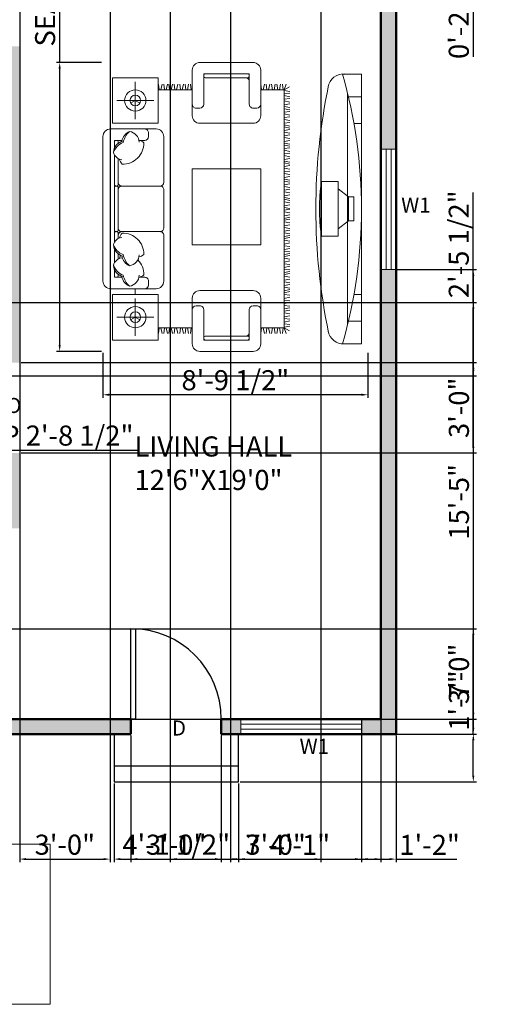
# Model space of a CAD drawing. Units: inches. Extents: x 3655 to 4051, y 2160 to 2854.
# Tile 2 of 3: x 3863 to 4051, y 2160 to 2552. Entities that reach past the tile are written whole.
import ezdxf

# ---------------------------------------------------------------- set-up
doc = ezdxf.new("R2010")
doc.units = ezdxf.units.IN
for name, color, linetype, lineweight in [('A-ANNO-DIMS', 2, 'Continuous', 18), ('A-ANNO-SCHD', 7, 'Continuous', 18), ('A-ANNO-TEXT', 7, 'Continuous', 18), ('A-AREA-IDEN', 7, 'Continuous', 25), ('A-DOOR', 3, 'Continuous', 25), ('A-FLOR-STRS', 7, 'Continuous', 25), ('A-FURN', 8, 'Continuous', 18), ('A-GLAZ', 4, 'Continuous', 18), ('A-WALL', 7, 'Continuous', 50)]:
    doc.layers.add(name, color=color, linetype=linetype, lineweight=lineweight)
doc.layers.add('A-WALL-PATT', color=244, linetype='Continuous', lineweight=13, true_color=0x991b1e)
doc.styles.get("Standard").update_dxf_attribs({"font": 'arial.ttf'})
doc.dimstyles.new('ISO-25', dxfattribs={"dimtxt": 8, "dimasz": 2.5, "dimexe": 1.25, "dimexo": 0.625, "dimtad": 1, "dimdec": 1, "dimlunit": 3, "dimtxsty": 'Standard', "dimcen": 2.5, "dimadec": 0, "dimazin": 0, "dimtfac": 1, "dimtdec": 1, "dimtmove": 0, "dimatfit": 3, "dimfxl": 1, "dimarcsym": 0})

# ---------------------------------------------------------------- blocks, each defined once
blk = doc.blocks.new('*U2')
for p, q in [((0, 0), (0, -6)), ((36, 0), (36, -6))]:
    blk.add_line(p, q)
blk.add_lwpolyline([(0, 0), (0, 36), (1.75, 36), (1.75, 0)], close=True)
blk.add_arc((0, 0), 36, 0, 90)
blk = doc.blocks.new('A$C78AE5658')
for p, q in [((925, 3400), (2825, 3400)), ((150, 3275), (150, 2675)), ((750, 3275), (150, 3275)), ((750, 2675), (750, 3275)), ((825, 2700), (825, 3300)), ((975, 3250), (975, 3152)), ((1080, 3250), (975, 3250)), ((995, 3250), (1080, 3250)), ((1163, 3250), (1350, 3250)), ((1350, 3250), (1163, 3250)), ((2587, 3250), (1433, 3250)), ((1433, 3250), (1555, 3250)), ((1595, 3250), (2155, 3250)), ((2587, 3250), (2195, 3250)), ((2775, 3250), (2670, 3250)), ((2755, 3250), (2670, 3250)), ((2775, 3152), (2775, 3250)), ((2925, 3300), (2925, 2700)), ((3000, 3275), (3000, 2675)), ((3600, 3275), (3000, 3275)), ((3600, 2675), (3600, 3275)), ((450, 2730), (450, 3220)), ((975, 3220), (975, 3230)), ((1013, 3200), (995, 3200)), ((1283, 3200), (1214, 3200)), ((1555, 3200), (1483, 3200)), ((1575, 3230), (1575, 3220)), ((1575, 3220), (1575, 3230)), ((1575, 3150), (1575, 2650)), ((2155, 3200), (1595, 3200)), ((2175, 3230), (2175, 3220)), ((2175, 3230), (2175, 3220)), ((2175, 3150), (2175, 2650)), ((2195, 3200), (2536, 3200)), ((2737, 3200), (2755, 3200)), ((2775, 3220), (2775, 3230)), ((3300, 2730), (3300, 3220)), ((450, 2975), (415, 3036)), ((3300, 2975), (3265, 3036)), ((205, 2975), (695, 2975)), ((450, 2975), (415, 2914)), ((750, 2975), (825, 2975)), ((975, 2927), (975, 2850)), ((2775, 2850), (2775, 2927)), ((3055, 2975), (3545, 2975)), ((3300, 2975), (3265, 2914)), ((925, 2800), (875, 2800)), ((2875, 2800), (2825, 2800)), ((150, 2675), (750, 2675)), ((308, 2659), (234, 2670)), ((308, 2637), (234, 2622)), ((308, 2589), (234, 2600)), ((308, 2675), (308, 2225)), ((1525, 2600), (925, 2600)), ((2125, 2600), (1625, 2600)), ((2825, 2600), (2225, 2600)), ((3000, 2675), (3600, 2675)), ((3442, 2675), (3442, 2225)), ((3442, 2659), (3516, 2670)), ((3442, 2637), (3516, 2622)), ((3442, 2589), (3516, 2600)), ((308, 2567), (234, 2552)), ((308, 2524), (234, 2535)), ((308, 2501), (234, 2487)), ((308, 2453), (234, 2464)), ((3442, 2567), (3516, 2552)), ((3442, 2524), (3516, 2535)), ((3442, 2501), (3516, 2487)), ((3442, 2453), (3516, 2464)), ((308, 2431), (234, 2417)), ((308, 2380), (234, 2391)), ((308, 2357), (234, 2343)), ((3442, 2431), (3516, 2417)), ((3442, 2380), (3516, 2391)), ((3442, 2357), (3516, 2343)), ((100, 2225), (700, 2225)), ((308, 2310), (234, 2321)), ((308, 2288), (234, 2273)), ((308, 2238), (234, 2249)), ((1400, 2225), (1400, 1325)), ((2400, 2225), (1400, 2225)), ((2400, 1325), (2400, 2225)), ((3700, 2225), (3100, 2225)), ((3442, 2310), (3516, 2321)), ((3442, 2288), (3516, 2273)), ((3442, 2238), (3516, 2249)), ((0, 1425), (0, 2125)), ((150, 2075), (150, 1475)), ((550, 2075), (150, 2075)), ((180, 2075), (170, 2075)), ((600, 2125), (600, 2175)), ((800, 2125), (800, 1425)), ((3000, 2125), (3000, 1425)), ((3200, 2125), (3200, 2175)), ((3250, 2075), (3650, 2075)), ((3620, 2075), (3630, 2075)), ((3650, 2075), (3650, 1475)), ((3800, 1425), (3800, 2125)), ((200, 2037), (200, 2055)), ((200, 1495), (200, 2037)), ((3600, 2037), (3600, 2055)), ((3600, 1495), (3600, 2037)), ((150, 1887), (150, 1495)), ((150, 1887), (150, 1475)), ((3650, 1887), (3650, 1495)), ((3650, 1887), (3650, 1475)), ((550, 1475), (150, 1475)), ((150, 1475), (550, 1475)), ((150, 1475), (550, 1475)), ((170, 1475), (180, 1475)), ((170, 1475), (180, 1475)), ((600, 1425), (600, 1375)), ((600, 1425), (600, 1375)), ((3200, 1425), (3200, 1375)), ((3200, 1425), (3200, 1375)), ((3250, 1475), (3650, 1475)), ((3650, 1475), (3250, 1475)), ((3650, 1475), (3250, 1475)), ((3630, 1475), (3620, 1475)), ((3630, 1475), (3620, 1475)), ((700, 1325), (100, 1325)), ((308, 1314), (234, 1325)), ((1400, 1325), (2400, 1325)), ((3100, 1325), (3700, 1325)), ((3442, 1314), (3516, 1325)), ((308, 1291), (234, 1277)), ((308, 1244), (234, 1255)), ((308, 1221), (234, 1207)), ((308, 1170), (234, 1181)), ((3442, 1291), (3516, 1277)), ((3442, 1244), (3516, 1255)), ((3442, 1221), (3516, 1207)), ((3442, 1170), (3516, 1181)), ((308, 1147), (234, 1133)), ((308, 1100), (234, 1111)), ((308, 1078), (234, 1063)), ((308, 1028), (234, 1039)), ((3442, 1147), (3516, 1133)), ((3442, 1100), (3516, 1111)), ((3442, 1078), (3516, 1063)), ((3442, 1028), (3516, 1039)), ((308, 1015), (236, 991)), ((308, 1015), (270, 946)), ((317, 1015), (332, 942)), ((363, 1015), (352, 942)), ((386, 1015), (400, 942)), ((434, 1015), (422, 942)), ((456, 1015), (470, 942)), ((507, 1015), (496, 942)), ((530, 1015), (544, 942)), ((559, 1015), (574, 942)), ((605, 1015), (594, 942)), ((628, 1015), (642, 942)), ((675, 1015), (664, 942)), ((698, 1015), (712, 942)), ((749, 1015), (738, 942)), ((771, 1015), (786, 942)), ((798, 1015), (813, 942)), ((845, 1015), (833, 942)), ((867, 1015), (881, 942)), ((915, 1015), (904, 942)), ((937, 1015), (951, 942)), ((989, 1015), (977, 942)), ((1011, 1015), (1025, 942)), ((1036, 1015), (1051, 942)), ((1082, 1015), (1071, 942)), ((1104, 1015), (1119, 942)), ((1152, 1015), (1141, 942)), ((1175, 1015), (1189, 942)), ((1226, 1015), (1215, 942)), ((1248, 1015), (1263, 942)), ((1273, 1015), (1287, 942)), ((1319, 1015), (1308, 942)), ((1341, 1015), (1355, 942)), ((1389, 1015), (1378, 942)), ((1411, 1015), (1426, 942)), ((1463, 1015), (1452, 942)), ((1485, 1015), (1499, 942)), ((1512, 1015), (1526, 942)), ((1558, 1015), (1547, 942)), ((1580, 1015), (1595, 942)), ((1628, 1015), (1617, 942)), ((1650, 1015), (1665, 942)), ((1702, 1015), (1691, 942)), ((1724, 1015), (1739, 942)), ((1750, 1015), (1764, 942)), ((1783, 1015), (1797, 942)), ((1834, 1015), (1823, 942)), ((1857, 1015), (1871, 942)), ((1894, 1015), (1879, 942)), ((1916, 1015), (1927, 942)), ((1967, 1015), (1953, 942)), ((2000, 1015), (1986, 942)), ((2026, 1015), (2012, 942)), ((2048, 1015), (2059, 942)), ((2100, 1015), (2085, 942)), ((2122, 1015), (2133, 942)), ((2170, 1015), (2155, 942)), ((2192, 1015), (2203, 942)), ((2238, 1015), (2224, 942)), ((2265, 1015), (2251, 942)), ((2288, 1015), (2299, 942)), ((2339, 1015), (2325, 942)), ((2361, 1015), (2372, 942)), ((2409, 1015), (2395, 942)), ((2431, 1015), (2443, 942)), ((2478, 1015), (2463, 942)), ((2502, 1015), (2487, 942)), ((2524, 1015), (2535, 942)), ((2576, 1015), (2561, 942)), ((2598, 1015), (2609, 942)), ((2646, 1015), (2631, 942)), ((2668, 1015), (2679, 942)), ((2714, 1015), (2700, 942)), ((2739, 1015), (2725, 942)), ((2762, 1015), (2773, 942)), ((2813, 1015), (2799, 942)), ((2835, 1015), (2847, 942)), ((2883, 1015), (2869, 942)), ((2906, 1015), (2917, 942)), ((2952, 1015), (2937, 942)), ((2979, 1015), (2964, 942)), ((3001, 1015), (3012, 942)), ((3052, 1015), (3038, 942)), ((3075, 1015), (3086, 942)), ((3123, 1015), (3108, 942)), ((3145, 1015), (3156, 942)), ((3191, 1015), (3177, 942)), ((3221, 1015), (3206, 942)), ((3243, 1015), (3254, 942)), ((3294, 1015), (3280, 942)), ((3317, 1015), (3328, 942)), ((3365, 1015), (3350, 942)), ((3387, 1015), (3398, 942)), ((3433, 1015), (3418, 942)), ((3442, 1015), (3515, 991)), ((3442, 1015), (3480, 946)), ((1515, 306), (1515, 524)), ((1515, 524), (2236, 524)), ((2236, 306), (2236, 524)), ((1515, 306), (2236, 306)), ((1613, 306), (1716, 168)), ((2137, 306), (2034, 168)), ((98, 250), (98, 252)), ((98, 250), (98, 0)), ((348, 184), (3398, 184)), ((398, 0), (398, 172)), ((2034, 168), (1716, 168)), ((1716, 168), (1716, 98)), ((2034, 168), (2034, 98)), ((3348, 0), (3348, 172)), ((3648, 250), (3648, 252)), ((3648, 0), (3648, 250)), ((3648, 0), (98, 0)), ((748, 0), (748, 99)), ((2034, 98), (1716, 98)), ((2998, 0), (2998, 99))]:
    blk.add_line(p, q)
for points in [[(308, 1325), (308, 1015), (1875, 1015)], [(3442, 1325), (3442, 1015), (1875, 1015)]]:
    blk.add_lwpolyline(points)
blk.add_lwpolyline([(246, 432, -0.103184), (3500, 432, -0.103184)], format="xyb")
for centre, radius in [((450, 2975), 140), ((3300, 2975), 140), ((450, 2975), 70), ((3300, 2975), 70)]:
    blk.add_circle(centre, radius)
for centre, radius, start, end in [((925, 3300), 100, 90, 180), ((2825, 3300), 100, 0, 90), ((995, 3230), 20, 90, 180), ((1145, 3093), 170, 94.5332, 162.7286), ((1209, 3055), 221, 110.2594, 158.4317), ((1100, 3136), 130, 7.768, 75.8936), ((1415, 3093), 170, 94.5332, 162.7286), ((1478, 3055), 221, 110.2594, 158.4317), ((1370, 3136), 130, 7.768, 75.8936), ((1555, 3230), 20, 0, 90), ((1595, 3230), 20, 90, 180), ((2155, 3230), 20, 0, 90), ((2195, 3230), 20, 90, 180), ((2650, 3136), 130, 104.1064, 172.232), ((2542, 3055), 221, 21.5683, 69.7406), ((2605, 3093), 170, 17.2714, 85.4668), ((2755, 3230), 20, 0, 90), ((1019, 2980), 177, 100.6387, 156.6848), ((1072, 2852), 293, 103.6492, 137.2632), ((995, 3220), 20, 180, 270), ((1289, 2980), 177, 100.6387, 156.6848), ((1342, 2852), 293, 103.6492, 137.2632), ((1173, 3032), 162, 56.7787, 73.2207), ((1278, 3140), 278, 269.4211, 1.715), ((1443, 3032), 162, 45.5055, 73.2207), ((1525, 3150), 50, 0, 90), ((1555, 3220), 20, 270, 0), ((1595, 3220), 20, 180, 270), ((1625, 3150), 50, 90, 180), ((2125, 3150), 50, 0, 90), ((2155, 3220), 20, 270, 0), ((2195, 3220), 20, 180, 270), ((2225, 3150), 50, 90, 180), ((2577, 3032), 162, 106.7793, 134.4945), ((2741, 3140), 278, 178.285, 270.5789), ((2678, 2852), 293, 42.7368, 76.3508), ((2755, 3220), 20, 270, 0), ((2731, 2980), 177, 23.3152, 79.3613), ((1006, 3075), 151, 189.3928, 267.9328), ((1275, 3075), 151, 189.3928, 267.9328), ((2745, 3075), 151, 272.0672, 350.6072), ((875, 2850), 50, 180, 270), ((925, 2850), 50, 270, 0), ((1088, 2940), 113, 186.2903, 223.8884), ((1009, 3140), 278, 269.4211, 314.7117), ((1357, 2940), 113, 186.2903, 223.8884), ((2663, 2940), 113, 316.1116, 353.7097), ((2825, 2850), 50, 180, 270), ((2875, 2850), 50, 270, 0), ((925, 2700), 100, 180, 270), ((1525, 2650), 50, 270, 0), ((1625, 2650), 50, 180, 270), ((2125, 2650), 50, 270, 0), ((2225, 2650), 50, 180, 270), ((2825, 2700), 100, 270, 0), ((100, 2125), 100, 90, 180), ((550, 2175), 50, 0, 90), ((700, 2125), 100, 0, 90), ((3100, 2125), 100, 90, 180), ((3250, 2175), 50, 90, 180), ((3700, 2125), 100, 0, 90), ((170, 2055), 20, 90, 180), ((180, 2055), 20, 0, 90), ((550, 2125), 50, 270, 0), ((3250, 2125), 50, 180, 270), ((3620, 2055), 20, 90, 180), ((3630, 2055), 20, 0, 90), ((100, 1425), 100, 180, 270), ((170, 1495), 20, 180, 270), ((180, 1495), 20, 270, 0), ((250, 1525), 50, 180, 270), ((550, 1425), 50, 0, 90), ((550, 1425), 50, 0, 90), ((700, 1425), 100, 270, 0), ((3100, 1425), 100, 180, 270), ((3250, 1425), 50, 90, 180), ((3250, 1425), 50, 90, 180), ((3550, 1525), 50, 270, 0), ((3620, 1495), 20, 180, 270), ((3630, 1495), 20, 270, 0), ((3700, 1425), 100, 270, 0), ((550, 1375), 50, 270, 0), ((550, 1375), 50, 270, 0), ((3250, 1375), 50, 180, 270), ((3250, 1375), 50, 180, 270), ((1875, -1675), 2228, 80.6925, 99.3075), ((298, 239), 200, 98.4687, 183.693), ((3449, 239), 200, 356.307, 81.5313), ((1873, 6426), 6426, 253.9658, 286.0342)]:
    blk.add_arc(centre, radius, start, end)
blk = doc.blocks.new('WIN-W1-48IN')
for p, q in [((0, 0), (0, 6)), ((48, 4), (0, 4)), ((48, 0), (48, 6)), ((48, 2), (0, 2))]:
    blk.add_line(p, q)
blk = doc.blocks.new('*D20')
at = {"layer": 'A-ANNO-DIMS', "color": 0, "lineweight": -2, "transparency": 16777216}
for p, q in [((3775.19, 2376.57), (3775.19, 2382.07)), ((3807.66, 2376.57), (3807.66, 2382.07)), ((3777.69, 2380.82), (3805.16, 2380.82)), ((3807.66, 2380.82), (3910.22, 2380.82))]:
    blk.add_line(p, q, dxfattribs=at)
at = {"layer": 'A-ANNO-DIMS', "color": 0, "transparency": 16777216}
for points in [[(3777.69, 2381.24), (3777.69, 2380.4), (3775.19, 2380.82)], [(3805.16, 2381.24), (3805.16, 2380.4), (3807.66, 2380.82)]]:
    blk.add_solid(points, dxfattribs=at)
at = {"layer": 'Defpoints', "color": 0, "transparency": 16777216}
for p in [(3807.66, 2380.82), (3775.19, 2375.95), (3807.66, 2375.95)]:
    blk.add_point(p, dxfattribs=at)
at = {"layer": 'A-ANNO-DIMS', "color": 0, "transparency": 16777216, "insert": (3860.19, 2385.58), "char_height": 8, "attachment_point": 5}
blk.add_mtext('COOKTOP 2\'-8 1/2"', dxfattribs=at)
blk = doc.blocks.new('*D22')
at = {"layer": 'A-ANNO-DIMS', "color": 0, "lineweight": -2, "transparency": 16777216}
for p, q in [((3879.35, 2535.27), (3879.35, 2656.5)), ((3895.99, 2535.27), (3878.1, 2535.27)), ((3879.35, 2422.65), (3879.35, 2532.77)), ((3895.99, 2420.15), (3878.1, 2420.15))]:
    blk.add_line(p, q, dxfattribs=at)
at = {"layer": 'A-ANNO-DIMS', "color": 0, "transparency": 16777216}
for points in [[(3878.93, 2532.77), (3879.76, 2532.77), (3879.35, 2535.27)], [(3878.93, 2422.65), (3879.76, 2422.65), (3879.35, 2420.15)]]:
    blk.add_solid(points, dxfattribs=at)
at = {"layer": 'Defpoints', "color": 0, "transparency": 16777216}
for p in [(3879.35, 2535.27), (3896.61, 2535.27), (3896.61, 2420.15)]:
    blk.add_point(p, dxfattribs=at)
at = {"layer": 'A-ANNO-DIMS', "color": 0, "transparency": 16777216, "insert": (3874.58, 2597.13), "char_height": 8, "attachment_point": 5, "rotation": 90}
blk.add_mtext('SEATING GROUP 9\'-7"', dxfattribs=at)
blk = doc.blocks.new('*D23')
at = {"layer": 'A-ANNO-DIMS', "color": 0, "lineweight": -2, "transparency": 16777216}
for p, q in [((3896.61, 2419.52), (3896.61, 2401.63)), ((4002.13, 2419.52), (4002.13, 2401.63)), ((3999.63, 2402.88), (3899.11, 2402.88))]:
    blk.add_line(p, q, dxfattribs=at)
at = {"layer": 'A-ANNO-DIMS', "color": 0, "transparency": 16777216}
for points in [[(3899.11, 2403.3), (3899.11, 2402.46), (3896.61, 2402.88)], [(3999.63, 2403.3), (3999.63, 2402.46), (4002.13, 2402.88)]]:
    blk.add_solid(points, dxfattribs=at)
at = {"layer": 'Defpoints', "color": 0, "transparency": 16777216}
for p in [(3896.61, 2420.15), (4002.13, 2420.15), (3896.61, 2402.88)]:
    blk.add_point(p, dxfattribs=at)
at = {"layer": 'A-ANNO-DIMS', "color": 0, "transparency": 16777216, "insert": (3949.37, 2407.64), "char_height": 8, "attachment_point": 5}
blk.add_mtext('8\'-9 1/2"', dxfattribs=at)
blk = doc.blocks.new('*D26')
at = {"layer": 'A-ANNO-DIMS', "color": 0, "lineweight": -2, "transparency": 16777216}
for p, q in [((3923.41, 2637.07), (3923.41, 2216.63)), ((4007.41, 2637.07), (4007.41, 2216.63)), ((3925.91, 2217.88), (4004.91, 2217.88))]:
    blk.add_line(p, q, dxfattribs=at)
at = {"layer": 'A-ANNO-DIMS', "color": 0, "transparency": 16777216}
for points in [[(3925.91, 2218.3), (3925.91, 2217.47), (3923.41, 2217.88)], [(4004.91, 2218.3), (4004.91, 2217.47), (4007.41, 2217.88)]]:
    blk.add_solid(points, dxfattribs=at)
at = {"layer": 'Defpoints', "color": 0, "transparency": 16777216}
for p in [(3923.41, 2637.69), (4007.41, 2637.69), (4007.41, 2217.88)]:
    blk.add_point(p, dxfattribs=at)
at = {"layer": 'A-ANNO-DIMS', "color": 0, "transparency": 16777216, "insert": (3965.41, 2222.59), "char_height": 8, "attachment_point": 5}
blk.add_mtext('7\'-0"', dxfattribs=at)
blk = doc.blocks.new('*D28')
at = {"layer": 'A-ANNO-DIMS', "color": 0, "lineweight": -2, "transparency": 16777216}
for p, q in [((3947.41, 2577.07), (3947.41, 2216.63)), ((3983.41, 2577.07), (3983.41, 2216.63)), ((3949.91, 2217.88), (3980.91, 2217.88))]:
    blk.add_line(p, q, dxfattribs=at)
at = {"layer": 'A-ANNO-DIMS', "color": 0, "transparency": 16777216}
for points in [[(3949.91, 2218.3), (3949.91, 2217.47), (3947.41, 2217.88)], [(3980.91, 2218.3), (3980.91, 2217.47), (3983.41, 2217.88)]]:
    blk.add_solid(points, dxfattribs=at)
at = {"layer": 'Defpoints', "color": 0, "transparency": 16777216}
for p in [(3947.41, 2577.69), (3983.41, 2577.69), (3983.41, 2217.88)]:
    blk.add_point(p, dxfattribs=at)
at = {"layer": 'A-ANNO-DIMS', "color": 0, "transparency": 16777216, "insert": (3965.41, 2222.59), "char_height": 8, "attachment_point": 5}
blk.add_mtext('3\'-0"', dxfattribs=at)
blk = doc.blocks.new('*D32')
at = {"layer": 'A-ANNO-DIMS', "color": 0, "lineweight": -2, "transparency": 16777216}
for p, q in [((3864.03, 2415.69), (4045.46, 2415.69)), ((4044.21, 2382.19), (4044.21, 2413.19)), ((3864.03, 2379.69), (4045.46, 2379.69))]:
    blk.add_line(p, q, dxfattribs=at)
at = {"layer": 'A-ANNO-DIMS', "color": 0, "transparency": 16777216}
for points in [[(4043.79, 2413.19), (4044.63, 2413.19), (4044.21, 2415.69)], [(4043.79, 2382.19), (4044.63, 2382.19), (4044.21, 2379.69)]]:
    blk.add_solid(points, dxfattribs=at)
at = {"layer": 'Defpoints', "color": 0, "transparency": 16777216}
for p in [(3863.41, 2415.69), (4044.21, 2415.69), (3863.41, 2379.69)]:
    blk.add_point(p, dxfattribs=at)
at = {"layer": 'A-ANNO-DIMS', "color": 0, "transparency": 16777216, "insert": (4039.5, 2397.69), "char_height": 8, "attachment_point": 5, "rotation": 90}
blk.add_mtext('3\'-0"', dxfattribs=at)
blk = doc.blocks.new('*D33')
at = {"layer": 'A-ANNO-DIMS', "color": 0, "lineweight": -2, "transparency": 16777216}
for p, q in [((3907.77, 2267.07), (3907.77, 2216.63)), ((3943.77, 2267.07), (3943.77, 2216.63)), ((3910.27, 2217.88), (3941.27, 2217.88))]:
    blk.add_line(p, q, dxfattribs=at)
at = {"layer": 'A-ANNO-DIMS', "color": 0, "transparency": 16777216}
for points in [[(3910.27, 2218.3), (3910.27, 2217.47), (3907.77, 2217.88)], [(3941.27, 2218.3), (3941.27, 2217.47), (3943.77, 2217.88)]]:
    blk.add_solid(points, dxfattribs=at)
at = {"layer": 'Defpoints', "color": 0, "transparency": 16777216}
for p in [(3907.77, 2267.69), (3943.77, 2267.69), (3943.77, 2217.88)]:
    blk.add_point(p, dxfattribs=at)
at = {"layer": 'A-ANNO-DIMS', "color": 0, "transparency": 16777216, "insert": (3925.77, 2222.59), "char_height": 8, "attachment_point": 5}
blk.add_mtext('3\'-0"', dxfattribs=at)
blk = doc.blocks.new('*D36')
at = {"layer": 'A-ANNO-DIMS', "color": 0, "lineweight": -2, "transparency": 16777216}
for p, q in [((3999.59, 2267.07), (3999.59, 2216.63)), ((3950.6, 2248.06), (3950.6, 2216.63)), ((3953.1, 2217.88), (3997.09, 2217.88))]:
    blk.add_line(p, q, dxfattribs=at)
at = {"layer": 'A-ANNO-DIMS', "color": 0, "transparency": 16777216}
for points in [[(3953.1, 2218.3), (3953.1, 2217.47), (3950.6, 2217.88)], [(3997.09, 2218.3), (3997.09, 2217.47), (3999.59, 2217.88)]]:
    blk.add_solid(points, dxfattribs=at)
at = {"layer": 'Defpoints', "color": 0, "transparency": 16777216}
for p in [(3999.59, 2267.69), (3950.6, 2248.68), (3999.59, 2217.88)]:
    blk.add_point(p, dxfattribs=at)
at = {"layer": 'A-ANNO-DIMS', "color": 0, "transparency": 16777216, "insert": (3975.09, 2222.52), "char_height": 8, "attachment_point": 5}
blk.add_mtext('4\'-1"', dxfattribs=at)
blk = doc.blocks.new('*D37')
at = {"layer": 'A-ANNO-DIMS', "color": 0, "lineweight": -2, "transparency": 16777216}
for p, q in [((3999.59, 2273.07), (3999.59, 2216.63)), ((4013.41, 2267.07), (4013.41, 2216.63)), ((4002.09, 2217.88), (4010.91, 2217.88)), ((4013.41, 2217.88), (4037.67, 2217.88))]:
    blk.add_line(p, q, dxfattribs=at)
at = {"layer": 'A-ANNO-DIMS', "color": 0, "transparency": 16777216}
for points in [[(4002.09, 2218.3), (4002.09, 2217.47), (3999.59, 2217.88)], [(4010.91, 2218.3), (4010.91, 2217.47), (4013.41, 2217.88)]]:
    blk.add_solid(points, dxfattribs=at)
at = {"layer": 'Defpoints', "color": 0, "transparency": 16777216}
for p in [(3999.59, 2273.69), (4013.41, 2267.69), (4013.41, 2217.88)]:
    blk.add_point(p, dxfattribs=at)
at = {"layer": 'A-ANNO-DIMS', "color": 0, "transparency": 16777216, "insert": (4026.79, 2222.52), "char_height": 8, "attachment_point": 5}
blk.add_mtext('1\'-2"', dxfattribs=at)
blk = doc.blocks.new('*D42')
at = {"layer": 'A-ANNO-DIMS', "color": 0, "lineweight": -2, "transparency": 16777216}
for p, q in [((4014.03, 2452.75), (4045.46, 2452.75)), ((4044.21, 2450.25), (4044.21, 2270.19)), ((4014.03, 2267.69), (4045.46, 2267.69))]:
    blk.add_line(p, q, dxfattribs=at)
at = {"layer": 'A-ANNO-DIMS', "color": 0, "transparency": 16777216}
for points in [[(4043.79, 2450.25), (4044.63, 2450.25), (4044.21, 2452.75)], [(4043.79, 2270.19), (4044.63, 2270.19), (4044.21, 2267.69)]]:
    blk.add_solid(points, dxfattribs=at)
at = {"layer": 'Defpoints', "color": 0, "transparency": 16777216}
for p in [(4013.41, 2452.75), (4013.41, 2267.69), (4044.21, 2267.69)]:
    blk.add_point(p, dxfattribs=at)
at = {"layer": 'A-ANNO-DIMS', "color": 0, "transparency": 16777216, "insert": (4039.5, 2360.22), "char_height": 8, "attachment_point": 5, "rotation": 90}
blk.add_mtext('15\'-5"', dxfattribs=at)
blk = doc.blocks.new('*D43')
at = {"layer": 'A-ANNO-DIMS', "color": 0, "lineweight": -2, "transparency": 16777216}
for p, q in [((3901.01, 2248.06), (3901.01, 2216.63)), ((3950.6, 2248.06), (3950.6, 2216.63)), ((3903.51, 2217.88), (3948.1, 2217.88))]:
    blk.add_line(p, q, dxfattribs=at)
at = {"layer": 'A-ANNO-DIMS', "color": 0, "transparency": 16777216}
for points in [[(3903.51, 2218.3), (3903.51, 2217.47), (3901.01, 2217.88)], [(3948.1, 2218.3), (3948.1, 2217.47), (3950.6, 2217.88)]]:
    blk.add_solid(points, dxfattribs=at)
at = {"layer": 'Defpoints', "color": 0, "transparency": 16777216}
for p in [(3901.01, 2248.68), (3950.6, 2248.68), (3950.6, 2217.88)]:
    blk.add_point(p, dxfattribs=at)
at = {"layer": 'A-ANNO-DIMS', "color": 0, "transparency": 16777216, "insert": (3925.81, 2222.64), "char_height": 8, "attachment_point": 5}
blk.add_mtext('4\'-1 1/2"', dxfattribs=at)
blk = doc.blocks.new('*D44')
at = {"layer": 'A-ANNO-DIMS', "color": 0, "lineweight": -2, "transparency": 16777216}
for p, q in [((4044.21, 2267.69), (4044.21, 2291.95)), ((3951.22, 2267.69), (4045.46, 2267.69)), ((4044.21, 2251.18), (4044.21, 2265.19)), ((3951.22, 2248.68), (4045.46, 2248.68))]:
    blk.add_line(p, q, dxfattribs=at)
at = {"layer": 'A-ANNO-DIMS', "color": 0, "transparency": 16777216}
for points in [[(4043.79, 2265.19), (4044.63, 2265.19), (4044.21, 2267.69)], [(4043.79, 2251.18), (4044.63, 2251.18), (4044.21, 2248.68)]]:
    blk.add_solid(points, dxfattribs=at)
at = {"layer": 'Defpoints', "color": 0, "transparency": 16777216}
for p in [(3950.6, 2267.69), (4044.21, 2267.69), (3950.6, 2248.68)]:
    blk.add_point(p, dxfattribs=at)
at = {"layer": 'A-ANNO-DIMS', "color": 0, "transparency": 16777216, "insert": (4039.57, 2281.07), "char_height": 8, "attachment_point": 5, "rotation": 90}
blk.add_mtext('1\'-7"', dxfattribs=at)
blk = doc.blocks.new('*D46')
at = {"layer": 'A-ANNO-DIMS', "color": 0, "lineweight": -2, "transparency": 16777216}
for p, q in [((3840.03, 2309.69), (4045.46, 2309.69)), ((4044.21, 2276.19), (4044.21, 2307.19)), ((3840.03, 2273.69), (4045.46, 2273.69))]:
    blk.add_line(p, q, dxfattribs=at)
at = {"layer": 'A-ANNO-DIMS', "color": 0, "transparency": 16777216}
for points in [[(4043.79, 2307.19), (4044.63, 2307.19), (4044.21, 2309.69)], [(4043.79, 2276.19), (4044.63, 2276.19), (4044.21, 2273.69)]]:
    blk.add_solid(points, dxfattribs=at)
at = {"layer": 'Defpoints', "color": 0, "transparency": 16777216}
for p in [(3839.41, 2309.69), (4044.21, 2309.69), (3839.41, 2273.69)]:
    blk.add_point(p, dxfattribs=at)
at = {"layer": 'A-ANNO-DIMS', "color": 0, "transparency": 16777216, "insert": (4039.5, 2291.69), "char_height": 8, "attachment_point": 5, "rotation": 90}
blk.add_mtext('3\'-0"', dxfattribs=at)
blk = doc.blocks.new('*D47')
at = {"layer": 'A-ANNO-DIMS', "color": 0, "lineweight": -2, "transparency": 16777216}
for p, q in [((3863.41, 2637.07), (3863.41, 2216.63)), ((3899.41, 2637.07), (3899.41, 2216.63)), ((3865.91, 2217.88), (3896.91, 2217.88))]:
    blk.add_line(p, q, dxfattribs=at)
at = {"layer": 'A-ANNO-DIMS', "color": 0, "transparency": 16777216}
for points in [[(3865.91, 2218.3), (3865.91, 2217.47), (3863.41, 2217.88)], [(3896.91, 2218.3), (3896.91, 2217.47), (3899.41, 2217.88)]]:
    blk.add_solid(points, dxfattribs=at)
at = {"layer": 'Defpoints', "color": 0, "transparency": 16777216}
for p in [(3863.41, 2637.69), (3899.41, 2637.69), (3899.41, 2217.88)]:
    blk.add_point(p, dxfattribs=at)
at = {"layer": 'A-ANNO-DIMS', "color": 0, "transparency": 16777216, "insert": (3881.41, 2222.59), "char_height": 8, "attachment_point": 5}
blk.add_mtext('3\'-0"', dxfattribs=at)
blk = doc.blocks.new('*D51')
at = {"layer": 'A-ANNO-DIMS', "color": 0, "lineweight": -2, "transparency": 16777216}
for p, q in [((4044.21, 2588.92), (4044.21, 2591.42)), ((3739.7, 2586.42), (4045.46, 2586.42)), ((4044.21, 2586.42), (4044.21, 2583.69)), ((3798.03, 2583.69), (4045.46, 2583.69)), ((4044.21, 2581.19), (4044.21, 2537.53))]:
    blk.add_line(p, q, dxfattribs=at)
at = {"layer": 'A-ANNO-DIMS', "color": 0, "transparency": 16777216}
for points in [[(4043.79, 2588.92), (4044.63, 2588.92), (4044.21, 2586.42)], [(4043.79, 2581.19), (4044.63, 2581.19), (4044.21, 2583.69)]]:
    blk.add_solid(points, dxfattribs=at)
at = {"layer": 'Defpoints', "color": 0, "transparency": 16777216}
for p in [(3739.07, 2586.42), (3797.41, 2583.69), (4044.21, 2583.69)]:
    blk.add_point(p, dxfattribs=at)
at = {"layer": 'A-ANNO-DIMS', "color": 0, "transparency": 16777216, "insert": (4039.45, 2558.11), "char_height": 8, "attachment_point": 5, "rotation": 90}
blk.add_mtext('0\'-2 1/2"', dxfattribs=at)
blk = doc.blocks.new('*D53')
at = {"layer": 'A-ANNO-DIMS', "color": 0, "lineweight": -2, "transparency": 16777216}
for p, q in [((4044.21, 2439.69), (4044.21, 2483.48)), ((3738.03, 2439.69), (4045.46, 2439.69)), ((4044.21, 2412.89), (4044.21, 2437.19)), ((3727.77, 2410.39), (4045.46, 2410.39))]:
    blk.add_line(p, q, dxfattribs=at)
at = {"layer": 'A-ANNO-DIMS', "color": 0, "transparency": 16777216}
for points in [[(4043.79, 2437.19), (4044.63, 2437.19), (4044.21, 2439.69)], [(4043.79, 2412.89), (4044.63, 2412.89), (4044.21, 2410.39)]]:
    blk.add_solid(points, dxfattribs=at)
at = {"layer": 'Defpoints', "color": 0, "transparency": 16777216}
for p in [(3737.41, 2439.69), (4044.21, 2439.69), (3727.14, 2410.39)]:
    blk.add_point(p, dxfattribs=at)
at = {"layer": 'A-ANNO-DIMS', "color": 0, "transparency": 16777216, "insert": (4039.45, 2462.84), "char_height": 8, "attachment_point": 5, "rotation": 90}
blk.add_mtext('2\'-5 1/2"', dxfattribs=at)

msp = doc.modelspace()

# ---------------------------------------------------------------- hatches: boundary and pattern name
at = {"layer": 'A-WALL-PATT'}
h = msp.add_hatch(color=256, dxfattribs=at)
h.dxf.hatch_style = 1
h.paths.add_polyline_path([(3713.41, 2787.69), (3761.41, 2787.69), (3761.41, 2793.69), (3707.41, 2793.69), (3707.41, 2622.69), (3713.41, 2622.69), (3713.41, 2637.69), (3821.41, 2637.69), (3821.41, 2643.69), (3713.41, 2643.69)])
h.paths.add_polyline_path([(3863.41, 2787.69), (3911.41, 2787.69), (3911.41, 2793.69), (3809.41, 2793.69), (3809.41, 2787.69), (3857.41, 2787.69), (3857.41, 2637.69), (3863.41, 2637.69)])
h.paths.add_polyline_path([(4013.41, 2793.69), (3959.41, 2793.69), (3959.41, 2787.69), (4007.41, 2787.69), (4007.41, 2643.69), (3899.41, 2643.69), (3899.41, 2637.69), (3917.41, 2637.69), (3917.41, 2577.69), (3947.41, 2577.69), (3947.41, 2583.69), (3923.41, 2583.69), (3923.41, 2637.69), (4007.41, 2637.69), (4007.41, 2583.69), (3983.41, 2583.69), (3983.41, 2577.69), (4007.41, 2577.69), (4007.41, 2500.75), (4013.41, 2500.75)])
h.paths.add_polyline_path([(3863.41, 2583.69), (3803.41, 2583.69), (3803.41, 2607.69), (3797.41, 2607.69), (3797.41, 2583.69), (3713.41, 2583.69), (3713.41, 2598.69), (3707.41, 2598.69), (3707.41, 2535.69), (3713.41, 2535.69), (3713.41, 2577.69), (3863.41, 2577.69)])
h.paths.add_polyline_path([(3863.41, 2541.69), (3857.41, 2541.69), (3857.41, 2445.69), (3713.41, 2445.69), (3713.41, 2487.69), (3707.41, 2487.69), (3707.41, 2421.69), (3713.41, 2421.69), (3713.41, 2439.69), (3857.41, 2439.69), (3857.41, 2415.69), (3863.41, 2415.69)])
h.paths.add_polyline_path([(3863.41, 2379.69), (3857.41, 2379.69), (3857.41, 2355.69), (3713.41, 2355.69), (3713.41, 2373.69), (3707.41, 2373.69), (3707.41, 2267.69), (3907.77, 2267.69), (3907.77, 2273.69), (3713.41, 2273.69), (3713.41, 2349.69), (3863.41, 2349.69)])
h.paths.add_polyline_path([(3951.59, 2273.69), (3943.77, 2273.69), (3943.77, 2267.69), (3951.59, 2267.69)])
h.paths.add_polyline_path([(4013.41, 2452.75), (4007.41, 2452.75), (4007.41, 2273.69), (3999.59, 2273.69), (3999.59, 2267.69), (4013.41, 2267.69)])

# ---------------------------------------------------------------- linework, layer by layer
at = {"layer": 'A-ANNO-SCHD'}
msp.add_lwpolyline([(3795.04, 2223.88), (3875.6, 2223.88), (3875.6, 2160.04), (3795.04, 2160.04)], close=True, dxfattribs=at)
at = {"layer": 'A-FLOR-STRS'}
for p, q in [((3901.01, 2267.69), (3901.01, 2248.68)), ((3950.6, 2248.68), (3950.6, 2267.69)), ((3950.6, 2254.97), (3901.01, 2254.97)), ((3901.01, 2248.68), (3950.6, 2248.68))]:
    msp.add_line(p, q, dxfattribs=at)
at = {"layer": 'A-WALL'}
for p, q in [((4013.41, 2793.69), (4013.41, 2267.69)), ((4007.41, 2577.69), (4007.41, 2273.69)), ((3713.41, 2273.69), (3907.77, 2273.69)), ((3907.77, 2267.69), (3907.77, 2273.69)), ((3943.77, 2267.69), (3943.77, 2273.69)), ((3943.77, 2273.69), (4007.41, 2273.69)), ((3707.41, 2267.69), (3907.77, 2267.69)), ((3943.77, 2267.69), (4013.41, 2267.69))]:
    msp.add_line(p, q, dxfattribs=at)

# ---------------------------------------------------------------- block references
at = {"layer": 'A-DOOR'}
msp.add_blockref('*U2', (3907.77, 2273.69), dxfattribs=at)
at = {"layer": 'A-FURN', "xscale": 0.0302930240957292, "yscale": 0.0302930240957292, "zscale": 0.0302930240957292, "rotation": 89.99999999999999}
msp.add_blockref('A$C78AE5658', (3999.61, 2420.15), dxfattribs=at)
at = {"layer": 'A-GLAZ', "rotation": 270}
msp.add_blockref('WIN-W1-48IN', (4007.41, 2500.75), dxfattribs=at)
at = {"layer": 'A-GLAZ'}
msp.add_blockref('WIN-W1-48IN', (3951.59, 2267.69), dxfattribs=at)

# ---------------------------------------------------------------- texts
at = {"layer": 'A-ANNO-TEXT', "char_height": 6, "attachment_point": 1}
for s, insert in [('W1', (4015.45, 2481.45)), ('O', (3858.03, 2401.62)), ('D', (3924.07, 2273.11)), ('W1', (3974.97, 2265.82))]:
    msp.add_mtext_dynamic_manual_height_columns(s, width=13.8821, gutter_width=12.5, heights=[0], dxfattribs=dict(at, insert=insert))
at = {"layer": 'A-AREA-IDEN', "insert": (3909.15, 2386.28), "char_height": 8, "attachment_point": 1}
msp.add_mtext_dynamic_manual_height_columns('LIVING HALL\\P12\'6"X19\'0"', width=84.0989, gutter_width=12.5, heights=[0], dxfattribs=at)

# ---------------------------------------------------------------- dimensions: what is measured, and where the dimension line sits
at = {"layer": 'A-ANNO-DIMS'}
dim = msp.add_linear_dim(base=(3879.35, 2535.27), p1=(3896.61, 2420.15), p2=(3896.61, 2535.27), angle=90, text='SEATING GROUP <>', dimstyle='ISO-25', override={"dimdec": 1, "dimlfac": 1, "dimrnd": 0, "dimzin": 1, "dimdsep": 46, "dimlunit": 4, "dimfrac": 2}, dxfattribs=at)
dim.commit()
dim.dimension.update_dxf_attribs({"geometry": '*D22', "text_midpoint": (3874.58, 2597.13)})
for base, p1, p2, picture, middle in [((3899.41, 2217.88), (3863.41, 2637.69), (3899.41, 2637.69), '*D47', (3881.41, 2222.59)), ((4007.41, 2217.88), (3923.41, 2637.69), (4007.41, 2637.69), '*D26', (3965.41, 2222.59)), ((3983.41, 2217.88), (3947.41, 2577.69), (3983.41, 2577.69), '*D28', (3965.41, 2222.59)), ((4013.41, 2217.88), (3999.59, 2273.69), (4013.41, 2267.69), '*D37', (4026.79, 2222.52)), ((3943.77, 2217.88), (3907.77, 2267.69), (3943.77, 2267.69), '*D33', (3925.77, 2222.59)), ((3999.59, 2217.88), (3950.6, 2248.68), (3999.59, 2267.69), '*D36', (3975.09, 2222.52)), ((3950.6, 2217.88), (3901.01, 2248.68), (3950.6, 2248.68), '*D43', (3925.81, 2222.64))]:
    dim = msp.add_linear_dim(base=base, p1=p1, p2=p2, dimstyle='ISO-25', override={"dimdec": 1, "dimlfac": 1, "dimrnd": 0, "dimzin": 1, "dimdsep": 46, "dimlunit": 4, "dimfrac": 2}, dxfattribs=at)
    dim.commit()
    dim.dimension.update_dxf_attribs({"geometry": picture, "text_midpoint": middle})
for base, p1, p2, angle, picture, middle in [((4044.21, 2583.69), (3739.07, 2586.42), (3797.41, 2583.69), 90, '*D51', (4039.45, 2558.11)), ((4044.21, 2439.69), (3727.14, 2410.39), (3737.41, 2439.69), 90, '*D53', (4039.45, 2462.84)), ((4044.21, 2267.69), (4013.41, 2452.75), (4013.41, 2267.69), 90, '*D42', (4039.5, 2360.22)), ((3896.61, 2402.88), (4002.13, 2420.15), (3896.61, 2420.15), 180, '*D23', (3949.37, 2407.64)), ((4044.21, 2415.69), (3863.41, 2379.69), (3863.41, 2415.69), 90, '*D32', (4039.5, 2397.69)), ((4044.21, 2309.69), (3839.41, 2273.69), (3839.41, 2309.69), 90, '*D46', (4039.5, 2291.69)), ((4044.21, 2267.69), (3950.6, 2248.68), (3950.6, 2267.69), 90, '*D44', (4039.57, 2281.07))]:
    dim = msp.add_linear_dim(base=base, p1=p1, p2=p2, angle=angle, dimstyle='ISO-25', override={"dimdec": 1, "dimlfac": 1, "dimrnd": 0, "dimzin": 1, "dimdsep": 46, "dimlunit": 4, "dimfrac": 2}, dxfattribs=at)
    dim.commit()
    dim.dimension.update_dxf_attribs({"geometry": picture, "text_midpoint": middle})
dim = msp.add_linear_dim(base=(3807.66, 2380.82), p1=(3775.19, 2375.95), p2=(3807.66, 2375.95), text='COOKTOP <>', dimstyle='ISO-25', override={"dimdec": 1, "dimlfac": 1, "dimrnd": 0, "dimzin": 1, "dimdsep": 46, "dimlunit": 4, "dimfrac": 2}, dxfattribs=at)
dim.commit()
dim.dimension.update_dxf_attribs({"geometry": '*D20', "text_midpoint": (3860.19, 2385.58)})

doc.saveas('drawing.dxf')
